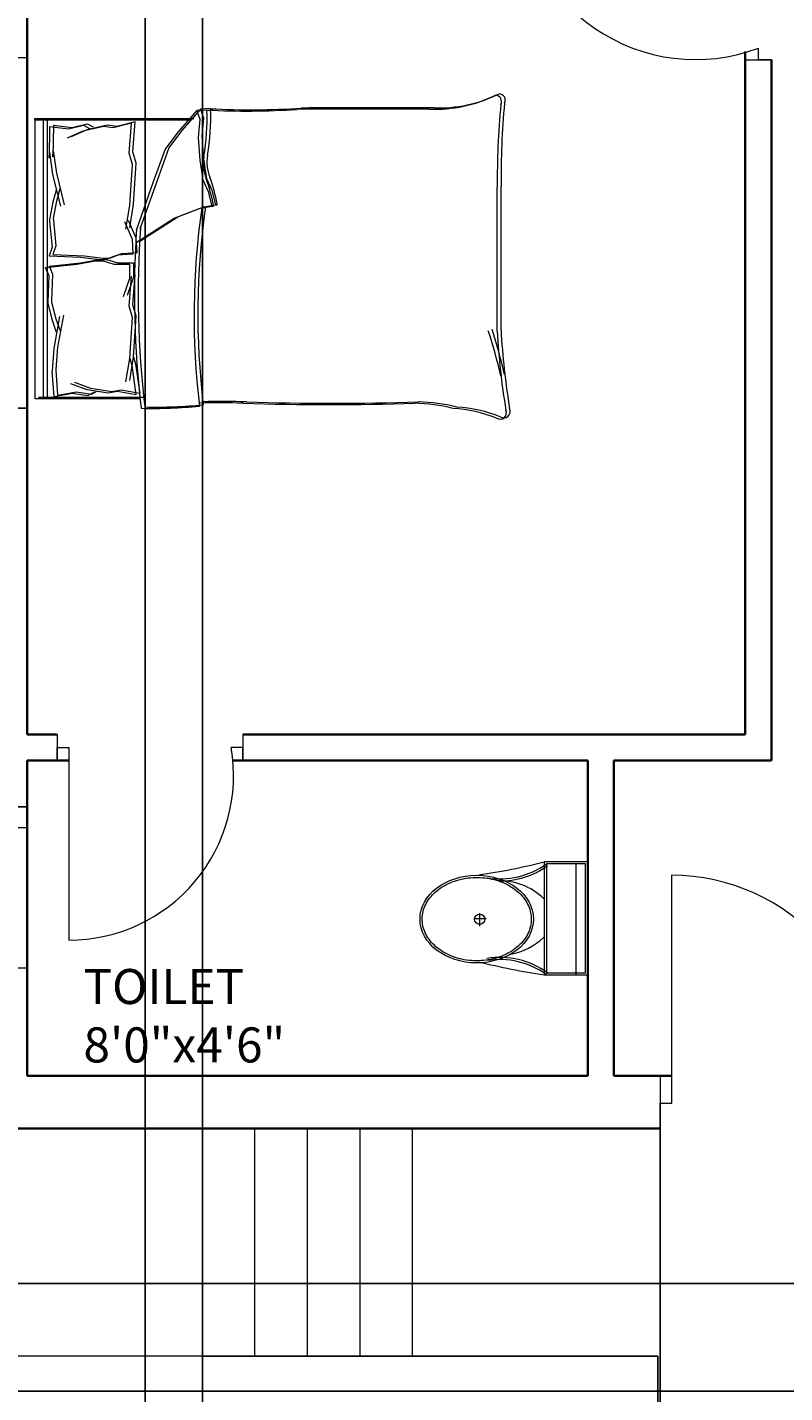
# Model space of a CAD drawing. Units: inches. Extents: x 1854 to 2495, y 1460 to 2772.
# Tile 8 of 12: x 1987 to 2117, y 1958 to 2192. Entities that reach past the tile are written whole.
import ezdxf

# ---------------------------------------------------------------- set-up
doc = ezdxf.new("R2010")
doc.units = ezdxf.units.IN
for name, color, linetype, lineweight in [('A-ANNO-DIMS', 2, 'Continuous', 18), ('A-AREA-IDEN', 7, 'Continuous', 18), ('A-DOOR', 3, 'Continuous', 18), ('A-EQPM-ELEV', 7, 'Continuous', 25), ('A-FLOR-FIXT', 9, 'Continuous', 18), ('A-FLOR-STRS', 7, 'Continuous', 18), ('A-FURN', 8, 'Continuous', 13), ('A-GLAZ', 4, 'Continuous', 18), ('A-WALL', 7, 'Continuous', 35)]:
    doc.layers.add(name, color=color, linetype=linetype, lineweight=lineweight)
doc.styles.get("Standard").update_dxf_attribs({"font": 'arial.ttf'})
doc.dimstyles.get("Standard").update_dxf_attribs({"dimtxt": 0.18, "dimasz": 0.18, "dimexe": 0.18, "dimexo": 0.0625, "dimgap": 0.09, "dimtad": 0, "dimtih": 1, "dimtoh": 1, "dimdec": 4, "dimzin": 0, "dimdsep": 46, "dimtxsty": 'Standard', "dimcen": 0.09, "dimadec": 0, "dimazin": 0, "dimtfac": 1, "dimtdec": 4, "dimtofl": 0, "dimtmove": 0, "dimatfit": 3, "dimfxl": 1, "dimtolj": 1, "dimtzin": 0, "dimarcsym": 0})

# ---------------------------------------------------------------- blocks, each defined once
blk = doc.blocks.new('A$C31115884')
for p, q in [((257.5, 466.4), (257.5, 523.2)), ((283.1, 497.7), (223.4, 497.7)), ((0, 200), (0, 0)), ((520, 200), (0, 200)), ((10, 190), (10, 10)), ((510, 190), (10, 190)), ((510, 10), (510, 190)), ((520, 0), (520, 200)), ((510, 54.5), (0, 54.5)), ((10, 10), (510, 10)), ((0, 0), (520, 0))]:
    blk.add_line(p, q)
blk.add_circle((255.6, 496.4), 23.6)
for centre, radius, start, end in [((2777.7, -204.6), 2807, 165.4549, 171.71327), ((-294.5, 403.3), 364.7, 324.20913, 9.34987), ((-294.5, 403.3), 374.7, 324.20913, 9.34987), ((805.8, 403.3), 364.7, 170.65013, 215.79087), ((3237, 905), 2807, 188.28673, 194.5451), ((139.5, 406.2), 293.5, 315.84364, 2.65635), ((805.8, 403.3), 374.7, 179.20365, 215.79087), ((383.6, 406.2), 293.5, 190.27735, 224.15636)]:
    blk.add_arc(centre, radius, start, end)
blk.add_ellipse((256.2, 509.9), major_axis=(0, -260.7), ratio=0.772727)
blk.add_open_spline([(256.2, 259.2), (263.1, 259.2), (270, 259.7), (287.8, 262.3), (298.7, 265.1), (319.9, 273.1), (330.2, 278.4), (350.1, 291.1), (359.7, 298.7), (377.7, 315.9), (386.2, 325.5), (401.7, 346.6), (408.8, 358.1), (421.3, 382.5), (426.8, 395.5), (435.9, 422.4), (439.5, 436.4), (444.8, 465.1), (446.5, 479.7), (447.9, 509.2), (447.6, 524), (445, 553.3), (442.7, 567.8), (436.3, 596), (432.1, 609.7), (421.9, 636), (416, 648.6), (402.5, 672.1), (395, 683), (378.6, 703), (369.8, 712.1), (351.1, 728), (341.3, 734.8), (320.9, 746.2), (310.4, 750.7), (288.9, 757.3), (278, 759.4), (256, 761), (245, 760.6), (223.1, 757.2), (212.3, 754.3), (191.1, 746.1), (180.8, 740.7), (160.9, 727.8), (151.4, 720.1), (133.5, 702.7), (125.1, 693), (109.6, 671.7), (102.6, 660.2), (90.2, 635.7), (84.9, 622.7), (76, 595.6), (72.4, 581.6), (67.2, 552.9), (65.6, 538.2), (64.4, 508.8), (64.8, 494), (67.5, 464.7), (69.9, 450.2), (76.6, 422), (80.8, 408.3), (91.1, 382.2), (97.2, 369.7), (110.8, 346.3), (118.4, 335.4), (134.8, 315.6), (143.7, 306.7), (162.4, 290.9), (172.3, 284.2), (192.8, 273), (203.3, 268.6), (224.8, 262.2), (235.8, 260.2), (249.9, 259.3), (253, 259.2), (256.2, 259.2)], degree=3, knots=[0, 0, 0, 0, 0.110105, 0.110105, 0.285049, 0.285049, 0.459994, 0.459994, 0.634938, 0.634938, 0.809882, 0.809882, 0.984827, 0.984827, 1.159771, 1.159771, 1.334715, 1.334715, 1.50966, 1.50966, 1.684604, 1.684604, 1.859549, 1.859549, 2.034493, 2.034493, 2.209437, 2.209437, 2.384382, 2.384382, 2.559326, 2.559326, 2.73427, 2.73427, 2.909215, 2.909215, 3.084159, 3.084159, 3.259103, 3.259103, 3.434048, 3.434048, 3.608992, 3.608992, 3.783936, 3.783936, 3.958881, 3.958881, 4.133825, 4.133825, 4.30877, 4.30877, 4.483714, 4.483714, 4.658658, 4.658658, 4.833603, 4.833603, 5.008547, 5.008547, 5.183491, 5.183491, 5.358436, 5.358436, 5.53338, 5.53338, 5.708324, 5.708324, 5.883269, 5.883269, 6.058213, 6.058213, 6.233158, 6.233158, 6.283185, 6.283185, 6.283185, 6.283185])
blk = doc.blocks.new('BED-DOUBLE')
for p, q in [((0, 51.27), (0, 51.49)), ((0, 51.49), (0.64, 51.49)), ((0.64, 51.49), (27.25, 51.49)), ((0.64, 51.49), (27.25, 51.49)), ((2.17, 3.7), (2.17, 51.49)), ((2.17, 3.7), (2.17, 51.49)), ((27.75, 52.87), (24.5, 49.16)), ((27.75, 52.87), (24.5, 49.16)), ((28.39, 53.1), (25.14, 49.39)), ((28.39, 53.1), (25.14, 49.39)), ((29.49, 52.95), (27.75, 52.87, 3.87)), ((29.49, 52.95), (27.75, 52.87, 3.87)), ((28.37, 51.33), (27.75, 52.87)), ((28.37, 51.33), (27.75, 52.87)), ((30.13, 53.18), (28.39, 53.1, 3.87)), ((30.13, 53.18), (28.39, 53.1, 3.87)), ((29, 51.56), (28.39, 53.1)), ((29, 51.56), (28.39, 53.1)), ((28.7, 48.46), (29, 51.56)), ((28.7, 48.46), (29, 51.56)), ((0, 51.27), (26.61, 51.27)), ((0, 51.27), (26.61, 51.27)), ((0, 51.27), (0, 3.48)), ((1.53, 3.48), (1.53, 51.27)), ((1.53, 3.48), (1.53, 51.27)), ((2.56, 50.11), (2.46, 44.71)), ((2.56, 50.11), (2.46, 44.71)), ((2.56, 50.11), (5.77, 49.73)), ((2.56, 50.11), (5.77, 49.73)), ((3.2, 50.34), (3.1, 44.94)), ((3.2, 50.34), (3.1, 44.94)), ((3.2, 50.34), (6.41, 49.96)), ((3.2, 50.34), (6.41, 49.96)), ((8.26, 49.31), (5.58, 48.13)), ((8.26, 49.31), (5.58, 48.13)), ((5.77, 49.73), (8.34, 50.33)), ((5.77, 49.73), (8.34, 50.33)), ((8.9, 49.54), (6.22, 48.36)), ((8.9, 49.54), (6.22, 48.36)), ((6.41, 49.96), (8.98, 50.56)), ((6.41, 49.96), (8.98, 50.56)), ((11.83, 50.11), (8.26, 49.31)), ((11.83, 50.11), (8.26, 49.31)), ((8.34, 50.33), (9.38, 49.81)), ((8.34, 50.33), (9.38, 49.81)), ((12.47, 50.34), (8.9, 49.54)), ((12.47, 50.34), (8.9, 49.54)), ((8.98, 50.56), (10.02, 50.04)), ((8.98, 50.56), (10.02, 50.04)), ((13.43, 49.92), (11.83, 50.11)), ((13.43, 49.92), (11.83, 50.11)), ((14.07, 50.15), (12.47, 50.34)), ((14.07, 50.15), (12.47, 50.34)), ((16.57, 50.7), (13.43, 49.92)), ((16.57, 50.7), (13.43, 49.92)), ((17.21, 50.93), (14.07, 50.15)), ((17.21, 50.93), (14.07, 50.15)), ((16.17, 45.57), (16.57, 50.7)), ((16.17, 45.57), (16.57, 50.7)), ((16.81, 45.8), (17.21, 50.93)), ((16.81, 45.79), (17.21, 50.93)), ((24.5, 49.16), (22.33, 46.22)), ((24.5, 49.16), (22.33, 46.22)), ((25.14, 49.39), (22.97, 46.45)), ((25.14, 49.39), (22.97, 46.45)), ((28.06, 48.23), (28.37, 51.33)), ((28.06, 48.23), (28.37, 51.33)), ((28.37, 44.36), (28.06, 48.23)), ((28.37, 44.36), (28.06, 48.23)), ((29, 44.59), (28.7, 48.46)), ((29, 44.59), (28.7, 48.46)), ((2.46, 44.71), (2.54, 45.71)), ((2.46, 44.71), (2.54, 45.71)), ((2.54, 45.71), (3.07, 41.91)), ((2.54, 45.71), (3.07, 41.91)), ((3.1, 44.94), (3.18, 45.94)), ((3.1, 44.94), (3.18, 45.94)), ((3.18, 45.94), (3.71, 42.14)), ((3.18, 45.94), (3.71, 42.14)), ((16.73, 43.61), (16.17, 45.57)), ((16.73, 43.61), (16.17, 45.57)), ((17.37, 43.83), (16.81, 45.8)), ((17.37, 43.83), (16.81, 45.79)), ((22.33, 46.22), (20.32, 40.64)), ((22.33, 46.22), (20.32, 40.64)), ((22.97, 46.45), (20.96, 40.87)), ((22.97, 46.45), (20.96, 40.87)), ((29.47, 41.18), (29, 44.59)), ((29.47, 41.18), (29, 44.59)), ((3.71, 42.14), (5.06, 36.72)), ((3.71, 42.14), (5.06, 36.72)), ((16.3, 36.6), (16.73, 43.61)), ((16.3, 36.6), (16.73, 43.61)), ((16.93, 36.82), (17.37, 43.83)), ((16.93, 36.82), (17.37, 43.83)), ((28.83, 40.95), (28.37, 44.36)), ((28.83, 40.95), (28.37, 44.36)), ((3.07, 41.91), (4.42, 36.5)), ((3.07, 41.91), (4.42, 36.5)), ((20.32, 40.64), (17.38, 32.31)), ((20.32, 40.64), (17.38, 32.31)), ((20.96, 40.87), (18.02, 32.53)), ((20.96, 40.87), (18.02, 32.53)), ((29.76, 38.94), (28.83, 40.95)), ((29.76, 38.94), (28.83, 40.95)), ((30.4, 39.17), (29.47, 41.18)), ((30.4, 39.17), (29.47, 41.18)), ((79.88, 15.29), (79.88, 39.91)), ((79.88, 15.29), (79.88, 39.91)), ((3.67, 39.2), (3.08, 37.14)), ((3.67, 39.2), (3.08, 37.14)), ((4.31, 39.43), (3.72, 37.36)), ((4.31, 39.43), (3.72, 37.36)), ((30.38, 36.46), (29.76, 38.94)), ((30.38, 36.46), (29.76, 38.94)), ((31.02, 36.69), (30.4, 39.17)), ((31.02, 36.69), (30.4, 39.17)), ((79.25, 15.06), (79.25, 39.68)), ((79.25, 15.06), (79.25, 39.68)), ((3.08, 37.14), (2.54, 34.2)), ((3.08, 37.14), (2.54, 34.2)), ((3.72, 37.36), (3.18, 34.43)), ((3.72, 37.36), (3.18, 34.43)), ((15.63, 32.56), (16.3, 36.6)), ((15.63, 32.56), (16.3, 36.6)), ((16.27, 32.79), (16.93, 36.82)), ((16.27, 32.79), (16.93, 36.82)), ((23.88, 34.45), (28.37, 36.15)), ((23.88, 34.45), (28.37, 36.15)), ((24.52, 34.68), (29, 36.38)), ((24.52, 34.68), (29, 36.38)), ((28.37, 36.15), (30.38, 36.46)), ((28.37, 36.15), (30.38, 36.46)), ((29, 36.38), (31.02, 36.69)), ((29, 36.38), (31.02, 36.69)), ((2.54, 34.2), (2.56, 33.88)), ((2.54, 34.2), (2.56, 33.88)), ((2.56, 33.88), (2.98, 29.46)), ((2.56, 33.88), (2.98, 29.46)), ((3.18, 34.43), (3.2, 34.11)), ((3.18, 34.43), (3.2, 34.11)), ((3.2, 34.11), (3.62, 29.68)), ((3.2, 34.11), (3.62, 29.68)), ((16.74, 30.75), (15.45, 33.82)), ((16.74, 30.75), (15.45, 33.82)), ((17.38, 30.98), (16.09, 34.05)), ((17.38, 30.98), (16.09, 34.05)), ((17.38, 30.26), (23.88, 34.45)), ((17.38, 30.26), (23.88, 34.45)), ((18.02, 30.49), (24.52, 34.68)), ((18.02, 30.49), (24.52, 34.68)), ((16.89, 28.3), (16.74, 30.75)), ((16.89, 28.3), (16.74, 30.75)), ((17.53, 28.53), (17.38, 30.98)), ((17.53, 28.53), (17.38, 30.98)), ((2.98, 29.46), (2.49, 27.98)), ((2.98, 29.46), (2.49, 27.98)), ((3.62, 29.68), (3.13, 28.21)), ((3.62, 29.68), (3.13, 28.21)), ((3.13, 28.21), (8.51, 27.96)), ((3.13, 28.21), (8.51, 27.96)), ((12.38, 27.44), (14.22, 28.13)), ((12.38, 27.44), (14.22, 28.13)), ((13.02, 27.66), (14.86, 28.36)), ((13.02, 27.66), (14.86, 28.36)), ((14.22, 28.13), (16.89, 28.3)), ((14.22, 28.13), (16.89, 28.3)), ((14.86, 28.36), (17.53, 28.53)), ((14.86, 28.36), (17.53, 28.53)), ((1.87, 25.98), (7.22, 26.56)), ((1.87, 25.98), (7.22, 26.56)), ((2.45, 24.54), (1.87, 25.98)), ((2.45, 24.54), (1.87, 25.98)), ((2.49, 27.98), (7.87, 27.73)), ((2.49, 27.98), (7.87, 27.73)), ((2.51, 26.21), (7.86, 26.79)), ((2.51, 26.21), (7.86, 26.79)), ((3.09, 24.77), (2.51, 26.21)), ((3.09, 24.77), (2.51, 26.21)), ((7.22, 26.56), (10.4, 27.14)), ((7.22, 26.56), (10.4, 27.14)), ((7.86, 26.79), (11.04, 27.37)), ((7.86, 26.79), (11.04, 27.37)), ((7.87, 27.73), (11.08, 27.36)), ((7.87, 27.73), (11.08, 27.35)), ((8.51, 27.96), (11.72, 27.58)), ((8.51, 27.96), (11.72, 27.58)), ((10.4, 27.14), (11.7, 27.14)), ((10.4, 27.14), (11.7, 27.14)), ((11.04, 27.37), (12.34, 27.37)), ((11.04, 27.37), (12.34, 27.37)), ((11.08, 27.36), (12.38, 27.44)), ((11.08, 27.35), (12.38, 27.44)), ((11.7, 27.14), (13.58, 26.56)), ((11.7, 27.14), (13.58, 26.56)), ((11.72, 27.58), (13.02, 27.66)), ((11.72, 27.58), (13.02, 27.66)), ((12.34, 27.37), (14.22, 26.79)), ((12.34, 27.37), (14.22, 26.79)), ((13.58, 26.56), (16.26, 26.56)), ((13.58, 26.56), (16.26, 26.56)), ((14.22, 26.79), (16.9, 26.79)), ((14.22, 26.79), (16.9, 26.79)), ((16.26, 26.56), (16.26, 24.1)), ((16.26, 26.56), (16.26, 24.1)), ((16.9, 26.79), (16.9, 24.33)), ((16.9, 26.79), (16.9, 24.33)), ((2.3, 20.09), (2.45, 24.54)), ((2.3, 20.09), (2.45, 24.54)), ((2.94, 20.32), (3.09, 24.77)), ((2.94, 20.32), (3.09, 24.77)), ((16.26, 24.1), (15.17, 20.96)), ((16.26, 24.1), (15.17, 20.96)), ((16.9, 24.33), (15.81, 21.19)), ((16.9, 24.33), (15.81, 21.19)), ((16.17, 19.38), (16.57, 24.52)), ((16.17, 19.38), (16.57, 24.52)), ((16.81, 19.61), (17.21, 24.74)), ((16.81, 19.61), (17.21, 24.74)), ((2.3, 19.77), (2.3, 20.09)), ((2.3, 19.77), (2.3, 20.09)), ((3.03, 16.88), (2.3, 19.77)), ((3.03, 16.88), (2.3, 19.77)), ((2.94, 20), (2.94, 20.32)), ((2.94, 20), (2.94, 20.32)), ((3.67, 17.11), (2.94, 20)), ((3.67, 17.11), (2.94, 20)), ((16.73, 17.42), (16.17, 19.38)), ((16.73, 17.42), (16.17, 19.38)), ((17.37, 17.65), (16.81, 19.61)), ((17.37, 17.65), (16.81, 19.61)), ((3.75, 14.86), (3.03, 16.88)), ((3.75, 14.85), (3.03, 16.88)), ((3.32, 12.11), (4.33, 17.6)), ((3.32, 12.11), (4.33, 17.6)), ((4.39, 15.08), (3.67, 17.11)), ((4.39, 15.08), (3.67, 17.11)), ((3.96, 12.34), (4.97, 17.83)), ((3.96, 12.34), (4.97, 17.83)), ((16.3, 10.41), (16.73, 17.42)), ((16.3, 10.41), (16.73, 17.42)), ((16.93, 10.64), (17.37, 17.65)), ((16.93, 10.64), (17.37, 17.65)), ((3.03, 8.29), (3.32, 12.11)), ((3.03, 8.28), (3.32, 12.11)), ((3.67, 8.51), (3.96, 12.34)), ((3.67, 8.51), (3.96, 12.34)), ((15.63, 6.38), (16.3, 10.41)), ((15.63, 6.38), (16.3, 10.41)), ((16.27, 6.61), (16.93, 10.64)), ((16.27, 6.61), (16.93, 10.64)), ((16.3, 10.41), (16.62, 9.28)), ((16.3, 10.41), (16.62, 9.28)), ((16.93, 10.64), (17.26, 9.51)), ((16.93, 10.64), (17.26, 9.51)), ((17.26, 9.51), (17.98, 4.41)), ((17.26, 9.51), (17.98, 4.41)), ((3.01, 8.18), (3.03, 8.29)), ((3.01, 8.18), (3.03, 8.28)), ((3.34, 3.9), (3.01, 8.18)), ((3.34, 3.9), (3.01, 8.18)), ((3.65, 8.41), (3.67, 8.51)), ((3.65, 8.41), (3.67, 8.51)), ((3.98, 4.13), (3.65, 8.41)), ((3.98, 4.13), (3.65, 8.41)), ((16.62, 9.28), (17.34, 4.18)), ((16.62, 9.28), (17.34, 4.18)), ((3.96, 4.12), (7.14, 4.7)), ((3.96, 4.12), (7.14, 4.7)), ((8.96, 5.05), (6.21, 6.06)), ((8.96, 5.05), (6.21, 6.06)), ((9.59, 5.28), (6.85, 6.29)), ((9.59, 5.28), (6.85, 6.29)), ((7.14, 4.7), (9.74, 4.27)), ((7.14, 4.7), (9.74, 4.27)), ((12.57, 4.47), (8.96, 5.05)), ((12.57, 4.47), (8.96, 5.05)), ((13.21, 4.7), (9.59, 5.28)), ((13.21, 4.7), (9.59, 5.28)), ((9.74, 4.27), (10.75, 4.85)), ((9.74, 4.27), (10.75, 4.85)), ((14.16, 4.76), (12.57, 4.47)), ((14.16, 4.76), (12.57, 4.47)), ((14.8, 4.99), (13.21, 4.7)), ((14.8, 4.99), (13.21, 4.7)), ((17.34, 4.18), (14.16, 4.76)), ((17.34, 4.18), (14.16, 4.76)), ((17.98, 4.41), (14.8, 4.99)), ((17.98, 4.41), (14.8, 4.99)), ((18.11, 3.48), (0, 3.48)), ((18.11, 3.48), (0, 3.48)), ((18.75, 3.7), (0.64, 3.7)), ((18.75, 3.7), (0.64, 3.7)), ((3.32, 3.89), (6.5, 4.47)), ((3.32, 3.89), (6.5, 4.47)), ((6.5, 4.47), (9.1, 4.04)), ((6.5, 4.47), (9.1, 4.04)), ((9.1, 4.04), (10.11, 4.62)), ((9.1, 4.04), (10.11, 4.62))]:
    blk.add_line(p, q)
for centre, radius, start, end in [((68.67, 76.16), 23.07, 267.4714, 296.4681), ((68.67, 76.16), 23.07, 267.4714, 296.4681), ((69.31, 76.39), 23.07, 267.4714, 296.4681), ((69.31, 76.39), 23.07, 267.4714, 296.4681), ((78.87, 54.41), 1.1, 332.6588, 86.02), ((78.87, 54.41), 1.1, 332.6588, 86.02), ((212.28, 41.15), 133.04, 174.4998, 180.6351), ((212.28, 41.15), 133.04, 174.4998, 180.6351), ((79.51, 54.64), 1.1, 332.6588, 86.02), ((79.51, 54.64), 1.1, 332.6588, 86.02), ((212.92, 41.38), 133.04, 174.4998, 180.6351), ((212.92, 41.38), 133.04, 174.4998, 180.6351), ((-6.66, 51.33), 36.18, 349.8763, 2.5657), ((-6.66, 51.33), 36.18, 349.8763, 2.5657), ((36.32, 182.27), 129.5, 266.9791, 273.8365), ((36.32, 182.27), 129.5, 266.9791, 273.8365), ((-6.02, 51.56), 36.18, 349.8763, 2.5657), ((-6.02, 51.56), 36.18, 349.8763, 2.5657), ((36.95, 182.49), 129.5, 266.9791, 273.8365), ((36.95, 182.49), 129.5, 266.9791, 273.8365), ((67.82, -4508.74), 4561.86, 90.00217, 90.28689), ((67.82, -4508.74), 4561.86, 90.00217, 90.28689), ((68.46, -4508.51), 4561.86, 90.00217, 90.28689), ((68.46, -4508.52), 4561.86, 90.00217, 90.28689), ((35.07, 43.74), 6.22, 168.6608, 203.7384), ((35.07, 43.74), 6.22, 168.6608, 203.7384), ((35.71, 43.97), 6.22, 168.6608, 203.7384), ((35.71, 43.97), 6.22, 168.6608, 203.7384), ((1.48, 31.15), 29.65, 10.6617, 19.8806), ((1.48, 31.15), 29.65, 10.6617, 19.8806), ((2.12, 31.38), 29.65, 10.6617, 19.8806), ((2.12, 31.38), 29.65, 10.6617, 19.8806), ((156.32, 17.76), 129.02, 171.7845, 186.9006), ((156.32, 17.76), 129.02, 171.7845, 186.9006), ((156.96, 17.98), 129.02, 171.7845, 186.9006), ((156.96, 17.98), 129.02, 171.7845, 186.9006), ((30.44, 36.64), 0.185, 250.2464, 1.1377), ((30.44, 36.64), 0.185, 250.2464, 1.1377), ((31.08, 36.86), 0.185, 250.2464, 1.1377), ((31.08, 36.86), 0.185, 250.2464, 1.1377), ((182.69, 21.59), 164.97, 176.0865, 186.7821), ((182.69, 21.59), 164.97, 176.0865, 186.7821), ((182.05, 21.36), 164.97, 176.0865, 186.7821), ((182.05, 21.36), 164.97, 176.0865, 186.7821), ((-23.71, -17.22), 106.46, 13.3832, 17.7053), ((-23.71, -17.22), 106.46, 13.3832, 17.7053), ((-23.07, -16.99), 106.46, 13.3832, 17.7053), ((-23.07, -16.99), 106.46, 13.3832, 17.7053), ((200.84, 21.43), 121.76, 182.9958, 189.4091), ((200.84, 21.43), 121.76, 182.9958, 189.4091), ((201.48, 21.66), 121.76, 182.9958, 189.4091), ((201.48, 21.66), 121.76, 182.9958, 189.4091), ((20.74, 85.39), 83.31, 268.7218, 275.604), ((20.74, 85.39), 83.31, 268.7218, 275.604), ((31.17, -167.31), 170.11, 88.4762, 91.0082), ((31.17, -167.31), 170.11, 88.4762, 91.0082), ((31.81, -167.08), 170.11, 88.4762, 91.0082), ((31.81, -167.08), 170.11, 88.4762, 91.0082), ((50.61, 484.82), 482.31, 268.2277, 271.7185), ((50.61, 484.82), 482.31, 268.2277, 271.7185), ((51.25, 485.05), 482.31, 268.2277, 271.7185), ((51.25, 485.05), 482.31, 268.2277, 271.7185), ((64.52, -26.9), 29.63, 76.0648, 88.9113), ((64.52, -26.9), 29.63, 76.0648, 88.9113), ((65.15, -26.67), 29.63, 76.0648, 88.9113), ((65.15, -26.67), 29.63, 76.0648, 88.9113), ((20.1, 85.16), 83.31, 268.7218, 275.604), ((20.1, 85.16), 83.31, 268.7218, 275.604), ((70.28, -21.66), 23.56, 67.9751, 86.652), ((70.28, -21.66), 23.56, 67.9751, 86.652), ((70.92, -21.43), 23.56, 67.9751, 86.652), ((70.92, -21.43), 23.56, 67.9751, 86.652), ((79.72, 1.09), 1.09, 236.1736, 23.4781), ((79.72, 1.09), 1.09, 236.1736, 23.4781), ((80.36, 1.32), 1.09, 236.1736, 23.4781), ((80.36, 1.32), 1.09, 236.1736, 23.4781)]:
    blk.add_arc(centre, radius, start, end)
blk = doc.blocks.new('WINDOW-60IN')
for p, q in [((0, 9), (0, 0)), ((60, 4.5), (60, 9)), ((60, 9), (60, 0)), ((0, 0), (0, 4.5)), ((0, 4.5), (60, 4.5))]:
    blk.add_line(p, q)
blk = doc.blocks.new('WINDOW-VENT-24IN')
for p, q in [((9, 24), (0, 24)), ((4.5, 24), (4.5, 0)), ((9, 0), (0, 0))]:
    blk.add_line(p, q)
blk = doc.blocks.new('*D36')
at = {"layer": 'A-ANNO-DIMS', "color": 0, "lineweight": -2, "transparency": 16777216}
for p, q in [((1977.98, 2054.59), (1977.98, 2058.31)), ((1978.16, 2058.13), (1982.02, 2058.13)), ((1986.8, 2058.13), (1982.94, 2058.13)), ((1986.98, 2054.59), (1986.98, 2058.31))]:
    blk.add_line(p, q, dxfattribs=at)
at = {"layer": 'A-ANNO-DIMS', "color": 0, "transparency": 16777216}
for points in [[(1978.16, 2058.16), (1978.16, 2058.1), (1977.98, 2058.13)], [(1986.8, 2058.16), (1986.8, 2058.1), (1986.98, 2058.13)]]:
    blk.add_solid(points, dxfattribs=at)
at = {"layer": 'Defpoints', "color": 0, "transparency": 16777216}
for p in [(1986.98, 2058.13), (1977.98, 2054.53), (1986.98, 2054.53)]:
    blk.add_point(p, dxfattribs=at)
at = {"layer": 'A-ANNO-DIMS', "color": 0, "transparency": 16777216, "insert": (1982.48, 2058.13), "char_height": 0.18, "attachment_point": 5}
blk.add_mtext('\\A1;9 TYP.', dxfattribs=at)
blk = doc.blocks.new('*D61')
at = {"layer": 'A-ANNO-DIMS', "color": 0, "lineweight": -2, "transparency": 16777216}
for p, q in [((1977.98, 1847.11), (1977.98, 2309.27)), ((1978.16, 2309.09), (1997.26, 2309.09)), ((2016.8, 2309.09), (1997.7, 2309.09)), ((2016.98, 1847.11), (2016.98, 2309.27))]:
    blk.add_line(p, q, dxfattribs=at)
at = {"layer": 'A-ANNO-DIMS', "color": 0, "transparency": 16777216}
for points in [[(1978.16, 2309.12), (1978.16, 2309.06), (1977.98, 2309.09)], [(2016.8, 2309.12), (2016.8, 2309.06), (2016.98, 2309.09)]]:
    blk.add_solid(points, dxfattribs=at)
at = {"layer": 'Defpoints', "color": 0, "transparency": 16777216}
for p in [(2016.98, 2309.09), (1977.98, 1847.04), (2016.98, 1847.04)]:
    blk.add_point(p, dxfattribs=at)
at = {"layer": 'A-ANNO-DIMS', "color": 0, "transparency": 16777216, "insert": (1997.48, 2309.09), "char_height": 0.18, "attachment_point": 5}
blk.add_mtext('\\A1;39', dxfattribs=at)
blk = doc.blocks.new('*D62')
at = {"layer": 'A-ANNO-DIMS', "color": 0, "lineweight": -2, "transparency": 16777216}
for p, q in [((2139.98, 2002.98), (2139.98, 1503.44)), ((2094.98, 1963.98), (2094.98, 1503.44)), ((2095.16, 1503.62), (2117.26, 1503.62)), ((2139.8, 1503.62), (2117.71, 1503.62))]:
    blk.add_line(p, q, dxfattribs=at)
at = {"layer": 'A-ANNO-DIMS', "color": 0, "transparency": 16777216}
for points in [[(2095.16, 1503.65), (2095.16, 1503.59), (2094.98, 1503.62)], [(2139.8, 1503.65), (2139.8, 1503.59), (2139.98, 1503.62)]]:
    blk.add_solid(points, dxfattribs=at)
at = {"layer": 'Defpoints', "color": 0, "transparency": 16777216}
for p in [(2139.98, 2003.04), (2094.98, 1964.04), (2139.98, 1503.62)]:
    blk.add_point(p, dxfattribs=at)
at = {"layer": 'A-ANNO-DIMS', "color": 0, "transparency": 16777216, "insert": (2117.48, 1503.62), "char_height": 0.18, "attachment_point": 5}
blk.add_mtext('\\A1;45', dxfattribs=at)
blk = doc.blocks.new('*D63')
at = {"layer": 'A-ANNO-DIMS', "color": 0, "lineweight": -2, "transparency": 16777216}
for p, q in [((1977.98, 2246.39), (1977.98, 1503.44)), ((2007.19, 2246.48), (2007.19, 1503.44)), ((1978.16, 1503.62), (1992.21, 1503.62)), ((2007.01, 1503.62), (1992.96, 1503.62))]:
    blk.add_line(p, q, dxfattribs=at)
at = {"layer": 'A-ANNO-DIMS', "color": 0, "transparency": 16777216}
for points in [[(1978.16, 1503.65), (1978.16, 1503.59), (1977.98, 1503.62)], [(2007.01, 1503.65), (2007.01, 1503.59), (2007.19, 1503.62)]]:
    blk.add_solid(points, dxfattribs=at)
at = {"layer": 'Defpoints', "color": 0, "transparency": 16777216}
for p in [(1977.98, 2246.45), (2007.19, 2246.54), (2007.19, 1503.62)]:
    blk.add_point(p, dxfattribs=at)
at = {"layer": 'A-ANNO-DIMS', "color": 0, "transparency": 16777216, "insert": (1992.59, 1503.62), "char_height": 0.18, "attachment_point": 5}
blk.add_mtext('\\A1;29.21', dxfattribs=at)
blk = doc.blocks.new('*D68')
at = {"layer": 'A-ANNO-DIMS', "color": 0, "lineweight": -2, "transparency": 16777216}
for p, q in [((2371.92, 1976.49), (1940.75, 1976.49)), ((1940.93, 1976.31), (1940.93, 1967.45)), ((1940.93, 1958.22), (1940.93, 1967.08)), ((2371.92, 1958.04), (1940.75, 1958.04))]:
    blk.add_line(p, q, dxfattribs=at)
at = {"layer": 'A-ANNO-DIMS', "color": 0, "transparency": 16777216}
for points in [[(1940.9, 1976.31), (1940.96, 1976.31), (1940.93, 1976.49)], [(1940.9, 1958.22), (1940.96, 1958.22), (1940.93, 1958.04)]]:
    blk.add_solid(points, dxfattribs=at)
at = {"layer": 'Defpoints', "color": 0, "transparency": 16777216}
for p in [(2371.98, 1976.49), (1940.93, 1958.04), (2371.98, 1958.04)]:
    blk.add_point(p, dxfattribs=at)
at = {"layer": 'A-ANNO-DIMS', "color": 0, "transparency": 16777216, "insert": (1940.93, 1967.27), "char_height": 0.18, "attachment_point": 5}
blk.add_mtext('\\A1;18.442', dxfattribs=at)
blk = doc.blocks.new('*D71')
at = {"layer": 'A-ANNO-DIMS', "color": 0, "lineweight": -2, "transparency": 16777216}
for p, q in [((2095.37, 2002.98), (2095.37, 1503.44)), ((2133.34, 2002.98), (2133.34, 1503.44)), ((2095.55, 1503.62), (2113.96, 1503.62)), ((2133.16, 1503.62), (2114.75, 1503.62))]:
    blk.add_line(p, q, dxfattribs=at)
at = {"layer": 'A-ANNO-DIMS', "color": 0, "transparency": 16777216}
for points in [[(2095.55, 1503.65), (2095.55, 1503.59), (2095.37, 1503.62)], [(2133.16, 1503.65), (2133.16, 1503.59), (2133.34, 1503.62)]]:
    blk.add_solid(points, dxfattribs=at)
at = {"layer": 'Defpoints', "color": 0, "transparency": 16777216}
for p in [(2095.37, 2003.04), (2133.34, 2003.04), (2133.34, 1503.62)]:
    blk.add_point(p, dxfattribs=at)
at = {"layer": 'A-ANNO-DIMS', "color": 0, "transparency": 16777216, "insert": (2114.36, 1503.62), "char_height": 0.18, "attachment_point": 5}
blk.add_mtext('\\A1;37.97', dxfattribs=at)

msp = doc.modelspace()

# ---------------------------------------------------------------- linework, layer by layer
at = {"layer": 'A-DOOR'}
for p, q in [((2112.2324, 2186.0549), (2112.2324, 2188.0549)), ((2109.9824, 2186.0549), (2114.4824, 2186.0549)), ((2114.4824, 2186.0549), (2112.2324, 2186.0549)), ((1992.0942, 2070.5449), (1992.0942, 2066.0449)), ((2023.918, 2070.5449), (2023.918, 2066.0449)), ((1992.0942, 2066.0449), (1992.0942, 2068.2949)), ((1992.0942, 2068.2949), (1992.0942, 2068.2949)), ((1992.0942, 2068.2949), (1994.0942, 2068.2949)), ((1994.0942, 2068.2949), (1994.0942, 2035.2949)), ((2023.918, 2068.2949), (2021.918, 2068.2949)), ((2023.918, 2066.0449), (2023.918, 2068.2949)), ((2097.3698, 2007.4023), (2097.3698, 2046.4023)), ((2095.3698, 2012.0449), (2095.3698, 2005.5239)), ((2095.3698, 2003.0449), (2095.3698, 2007.4023)), ((2095.3698, 2007.4023), (2097.3698, 2007.4023)), ((2095.3698, 2005.5239), (2095.3698, 2003.0449))]:
    msp.add_line(p, q, dxfattribs=at)
for centre, radius, start, end in [((2101.4541, 2216.5567), 30.4717, 180, 290.714797), ((1994.0942, 2063.5247), 28.2298, 270, 9.728371), ((2097.3698, 2012.1239), 34.2784, 352.32339, 90)]:
    msp.add_arc(centre, radius, start, end, dxfattribs=at)
at = {"layer": 'A-EQPM-ELEV'}
for p, q in [((2016.9824, 1964.0449), (2094.9824, 1964.0449)), ((2016.9824, 1964.0449), (2016.9824, 1886.0449)), ((2094.9824, 1943.9813), (2094.9824, 1964.0449))]:
    msp.add_line(p, q, dxfattribs=at)
at = {"layer": 'A-FLOR-STRS'}
for p, q in [((2016.9824, 1964.0449), (2016.9824, 2003.0449)), ((2025.9824, 1964.0449), (2025.9824, 2003.0449)), ((2034.9824, 1964.0449), (2034.9824, 2003.0449)), ((2043.9824, 1964.0449), (2043.9824, 2003.0449)), ((2052.9824, 1964.0449), (2052.9824, 2003.0449)), ((2016.9824, 1964.0449), (1977.9824, 1964.0449))]:
    msp.add_line(p, q, dxfattribs=at)
at = {"layer": 'A-WALL'}
for p, q in [((1986.9824, 2237.5449), (1986.9824, 2070.5449)), ((2109.9824, 2187.4934), (2109.9824, 2070.5449)), ((2114.4824, 2186.0549), (2114.4824, 2070.5449)), ((1986.9824, 2070.5449), (1992.0942, 2070.5449)), ((2023.918, 2070.5449), (2109.9824, 2070.5449)), ((2114.4824, 2070.5449), (2114.4824, 2066.0449)), ((1986.9824, 2066.0449), (1994.0942, 2066.0449)), ((1986.9824, 2066.0449), (1986.9824, 2012.0449)), ((1986.9824, 2066.0449), (1994.0942, 2066.0449)), ((2022.2112, 2066.0449), (2082.9824, 2066.0449)), ((2022.2112, 2066.0449), (2082.9824, 2066.0449)), ((2082.9824, 2066.0449), (2082.9824, 2012.0449)), ((2087.4824, 2012.0449), (2087.4824, 2066.0449)), ((2087.4824, 2066.0449), (2114.4824, 2066.0449)), ((1986.9824, 2012.0449), (2082.9824, 2012.0449)), ((2087.4824, 2012.0449), (2097.3698, 2012.0449)), ((1977.9824, 2003.0449), (2095.3698, 2003.0449))]:
    msp.add_line(p, q, dxfattribs=at)

# ---------------------------------------------------------------- block references
at = {"layer": 'A-FLOR-FIXT', "xscale": 0.0372717239612423, "yscale": 0.0372717239612423, "zscale": 0.0372717239612423, "rotation": 89.99999999999999}
msp.add_blockref('A$C31115884', (2082.9824, 2029.3543), dxfattribs=at)
at = {"layer": 'A-FURN'}
msp.add_blockref('BED-DOUBLE', (1988.253, 2124.507), dxfattribs=at)
at = {"layer": 'A-GLAZ', "rotation": 270.0000000000002}
msp.add_blockref('WINDOW-60IN', (1977.9825, 2186.3716), dxfattribs=at)
at = {"layer": 'A-GLAZ'}
msp.add_blockref('WINDOW-VENT-24IN', (1977.982, 2030.528), dxfattribs=at)

# ---------------------------------------------------------------- texts
at = {"layer": 'A-AREA-IDEN', "insert": (1996.6034, 2030.3611), "char_height": 6, "attachment_point": 1}
msp.add_mtext_dynamic_manual_height_columns('TOILET\\P8\'0"x4\'6"', width=66.01185, gutter_width=12.5, heights=[0], dxfattribs=at)

# ---------------------------------------------------------------- dimensions: what is measured, and where the dimension line sits
at = {"layer": 'A-ANNO-DIMS'}
for base, p1, p2, override, picture, middle in [((2016.9824, 2309.0949), (1977.9824, 1847.0449), (2016.9824, 1847.0449), {"dimdec": 0, "dimlfac": 1, "dimrnd": 0, "dimzin": 0, "dimdsep": 46, "dimlunit": 2}, '*D61', (1997.4824, 2309.0949)), ((2007.1898, 1503.6207), (1977.9824, 2246.45), (2007.1898, 2246.5449), {"dimdec": 2, "dimlfac": 1, "dimrnd": 0, "dimzin": 0, "dimdsep": 46, "dimlunit": 2}, '*D63', (1992.5861, 1503.6207)), ((2139.9824, 1503.6207), (2094.9824, 1964.0449), (2139.9824, 2003.0449), {"dimdec": 0, "dimlfac": 1, "dimrnd": 0, "dimzin": 0, "dimdsep": 46, "dimlunit": 2}, '*D62', (2117.4824, 1503.6207)), ((2133.341, 1503.6207), (2095.3698, 2003.0449), (2133.341, 2003.0449), {"dimdec": 2, "dimlfac": 1, "dimrnd": 0, "dimzin": 0, "dimdsep": 46, "dimlunit": 2}, '*D71', (2114.3554, 1503.6207))]:
    dim = msp.add_linear_dim(base=base, p1=p1, p2=p2, dimstyle='Standard', override=override, dxfattribs=at)
    dim.commit()
    dim.dimension.update_dxf_attribs({"geometry": picture, "text_midpoint": middle})
dim = msp.add_linear_dim(base=(1986.9824, 2058.1278), p1=(1977.9824, 2054.5278), p2=(1986.9824, 2054.5278), text='<> TYP.', dimstyle='Standard', override={"dimdec": 0, "dimlfac": 1, "dimrnd": 0, "dimzin": 0, "dimdsep": 46, "dimlunit": 2}, dxfattribs=at)
dim.commit()
dim.dimension.update_dxf_attribs({"geometry": '*D36', "text_midpoint": (1982.4824, 2058.1278)})
dim = msp.add_linear_dim(base=(1940.93239, 1958.04492), p1=(2371.98239, 1976.48735), p2=(2371.98239, 1958.04492), angle=90, dimstyle='Standard', override={"dimdec": 3, "dimlfac": 1, "dimrnd": 0, "dimzin": 0, "dimdsep": 46, "dimlunit": 2}, dxfattribs=at)
dim.commit()
dim.dimension.update_dxf_attribs({"geometry": '*D68', "text_midpoint": (1940.93239, 1967.26613)})

doc.saveas('drawing.dxf')
